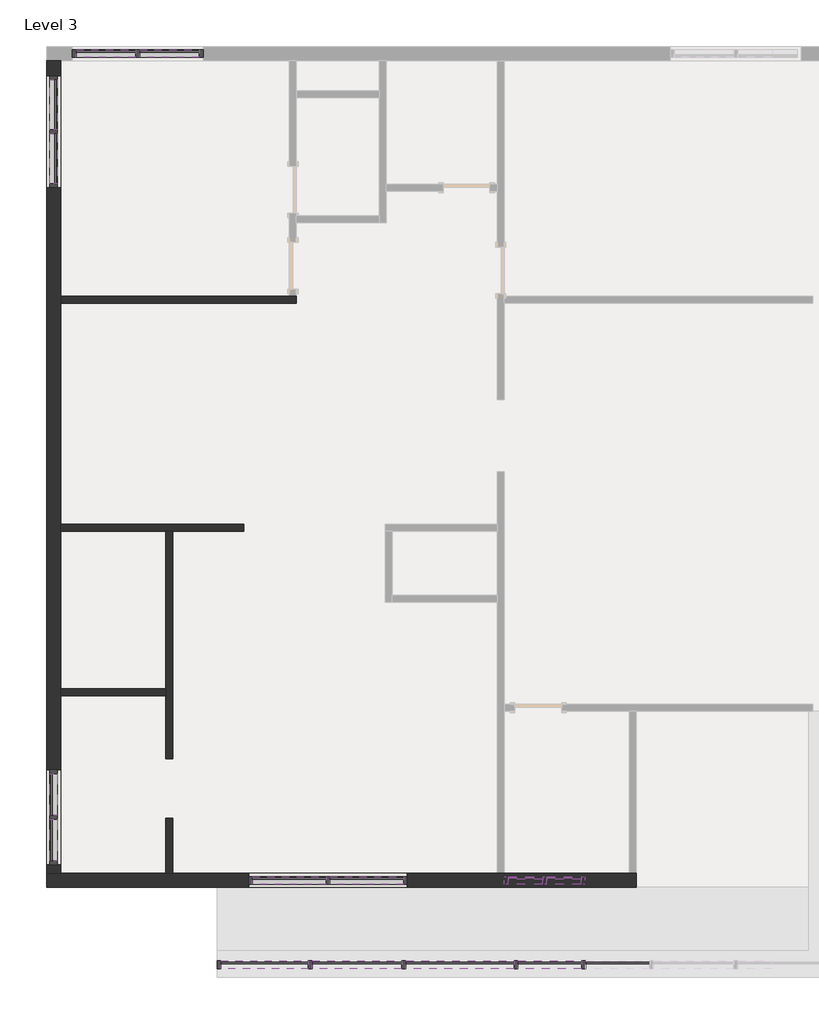
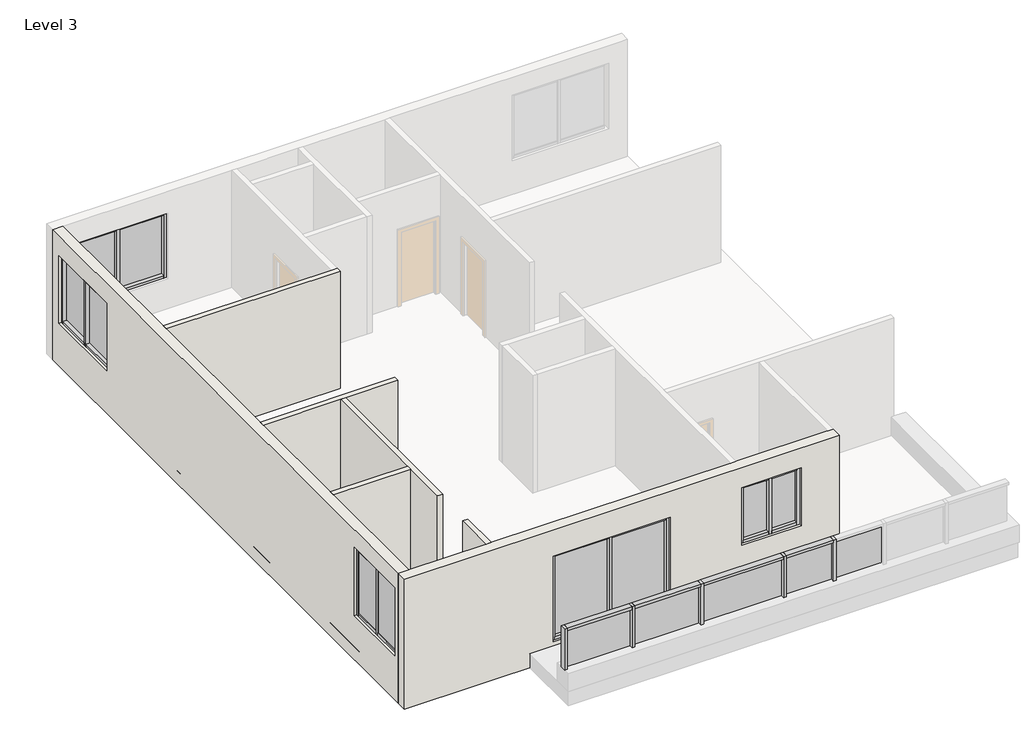
# One storey, part 1 of 2: 44 members, 15 plates, 7 walls.
"""IFC4 building model written with IfcOpenShell, lengths in millimetres."""

from ifc_helpers import new_model, si_unit, frame, origin, place, context, project, spatial, polyline, outline, extrude, faceted_brep, transform, mapped, element, save
from components import member_c17f1be2, member_801a2072, member_8e397d51, member_e9c7f4a4, member_4b34273c, member_2bcda102, member_43707fe5, member_d6231c0b, member_8613ee48, member_ea832cfd, member_e65a551c, member_6f41c4f0, member_2710255a, member_a910906a, member_01694e6c, member_4a1dde21, member_f8454dad, member_26d67f61, member_dda01c07, member_6d5c3e5e, member_04769ced, system_panel_glazed_e1e0096c, system_panel_glazed_c67bbfce, system_panel_glazed_bf6811db, system_panel_glazed_f54daf4a, system_panel_glazed_2cda0698, system_panel_glazed_7b3c61a9, system_panel_glazed_c86d0b30, system_panel_glazed_0021da76, system_panel_glazed_8b2f71d4

model = new_model("IFC4")

# Units and contexts
model_context = context("Model", 3, world=origin())
ifc_project = project(units=[si_unit("LENGTHUNIT", "METRE", prefix="MILLI")], contexts=[model_context])

# Site, building, storey
site = spatial("IfcSite", under=ifc_project)
building = spatial("IfcBuilding", under=site)
storey = spatial("IfcBuildingStorey", under=building, Name="Level 3", Elevation=6096.0)

# Members
placement = place(None, origin())
member_shape = member_c17f1be2(model_context)
element("IfcMember", 1, ObjectType="Rectangular Mullion : 2.5\" x 5\" rectangular", at=placement, inside=storey, context=model_context, shape_type="MappedRepresentation", body=[
    mapped(member_shape, transform((-18883.3195233, -1777.6752569, 8683.0746559), x_axis=(0.0, 0.0, 1.0), y_axis=(-1.0, 0.0, 0.0), z_axis=(0.0, -1.0, 0.0))),
])
element("IfcMember", 2, ObjectType="Rectangular Mullion : 2.5\" x 5\" rectangular", at=placement, inside=storey, context=model_context, shape_type="MappedRepresentation", body=[
    mapped(member_shape, transform((-18883.3195233, -2660.3252569, 8683.0746559), x_axis=(0.0, 0.0, 1.0), y_axis=(-1.0, 0.0, 0.0), z_axis=(0.0, -1.0, 0.0))),
])
element("IfcMember", 3, ObjectType="Rectangular Mullion : 2.5\" x 5\" rectangular", at=placement, inside=storey, context=model_context, shape_type="MappedRepresentation", body=[
    mapped(member_shape, transform((-18883.3195233, -1841.1752569, 7103.3616568), x_axis=(0.0, 0.0, -1.0), y_axis=(-1.0, 0.0, 0.0), z_axis=(0.0, 1.0, 0.0))),
])
element("IfcMember", 4, ObjectType="Rectangular Mullion : 2.5\" x 5\" rectangular", at=placement, inside=storey, context=model_context, shape_type="MappedRepresentation", body=[
    mapped(member_shape, transform((-18883.3195233, -958.5252569, 7103.3616568), x_axis=(0.0, 0.0, -1.0), y_axis=(-1.0, 0.0, 0.0), z_axis=(0.0, 1.0, 0.0))),
])
member_2_shape = member_801a2072(model_context)
element("IfcMember", 5, ObjectType="Rectangular Mullion : 2.5\" x 5\" rectangular", at=placement, inside=storey, context=model_context, shape_type="MappedRepresentation", body=[
    mapped(member_2_shape, transform((-17543.4695233, -533.0752569, 8635.8598955), x_axis=(0.0, 0.0, 1.0), y_axis=(0.0, -1.0, 0.0), z_axis=(1.0, 0.0, 0.0))),
])
element("IfcMember", 6, ObjectType="Rectangular Mullion : 2.5\" x 5\" rectangular", at=placement, inside=storey, context=model_context, shape_type="MappedRepresentation", body=[
    mapped(member_2_shape, transform((-16508.4195233, -533.0752569, 8635.8598955), x_axis=(0.0, 0.0, 1.0), y_axis=(0.0, -1.0, 0.0), z_axis=(1.0, 0.0, 0.0))),
])
element("IfcMember", 7, ObjectType="Rectangular Mullion : 2.5\" x 5\" rectangular", at=placement, inside=storey, context=model_context, shape_type="MappedRepresentation", body=[
    mapped(member_2_shape, transform((-17479.9695233, -533.0752569, 7102.6124164), x_axis=(0.0, 0.0, -1.0), y_axis=(0.0, -1.0, 0.0), z_axis=(-1.0, 0.0, 0.0))),
])
element("IfcMember", 8, ObjectType="Rectangular Mullion : 2.5\" x 5\" rectangular", at=placement, inside=storey, context=model_context, shape_type="MappedRepresentation", body=[
    mapped(member_2_shape, transform((-18515.0195233, -533.0752569, 7102.6124164), x_axis=(0.0, 0.0, -1.0), y_axis=(0.0, -1.0, 0.0), z_axis=(-1.0, 0.0, 0.0))),
])
member_3_shape = member_8e397d51(model_context)
element("IfcMember", 9, ObjectType="Rectangular Mullion : 2.5\" x 5\" rectangular", at=placement, inside=storey, context=model_context, shape_type="MappedRepresentation", body=[
    mapped(member_3_shape, transform((-10904.5445233, -14020.4752569, 8672.741835), x_axis=(0.0, 0.0, 1.0), y_axis=(0.0, -1.0, 0.0), z_axis=(1.0, 0.0, 0.0))),
])
element("IfcMember", 10, ObjectType="Rectangular Mullion : 2.5\" x 5\" rectangular", at=placement, inside=storey, context=model_context, shape_type="MappedRepresentation", body=[
    mapped(member_3_shape, transform((-10279.0695233, -14020.4752569, 8672.741835), x_axis=(0.0, 0.0, 1.0), y_axis=(0.0, -1.0, 0.0), z_axis=(1.0, 0.0, 0.0))),
])
element("IfcMember", 11, ObjectType="Rectangular Mullion : 2.5\" x 5\" rectangular", at=placement, inside=storey, context=model_context, shape_type="MappedRepresentation", body=[
    mapped(member_3_shape, transform((-10841.0445233, -14020.4752569, 7322.7664741), x_axis=(0.0, 0.0, -1.0), y_axis=(0.0, -1.0, 0.0), z_axis=(-1.0, 0.0, 0.0))),
])
element("IfcMember", 12, ObjectType="Rectangular Mullion : 2.5\" x 5\" rectangular", at=placement, inside=storey, context=model_context, shape_type="MappedRepresentation", body=[
    mapped(member_3_shape, transform((-11466.5195233, -14020.4752569, 7322.7664741), x_axis=(0.0, 0.0, -1.0), y_axis=(0.0, -1.0, 0.0), z_axis=(-1.0, 0.0, 0.0))),
])
member_4_shape = member_e9c7f4a4(model_context)
element("IfcMember", 13, ObjectType="Rectangular Mullion : 2.5\" x 5\" rectangular", at=placement, inside=storey, context=model_context, shape_type="MappedRepresentation", body=[
    mapped(member_4_shape, transform((-14438.3195233, -14020.4752569, 8530.8973501), x_axis=(0.0, 0.0, 1.0), y_axis=(0.0, -1.0, 0.0), z_axis=(1.0, 0.0, 0.0))),
])
element("IfcMember", 14, ObjectType="Rectangular Mullion : 2.5\" x 5\" rectangular", at=placement, inside=storey, context=model_context, shape_type="MappedRepresentation", body=[
    mapped(member_4_shape, transform((-13174.6695233, -14020.4752569, 8530.8973501), x_axis=(0.0, 0.0, 1.0), y_axis=(0.0, -1.0, 0.0), z_axis=(1.0, 0.0, 0.0))),
])
element("IfcMember", 15, ObjectType="Rectangular Mullion : 2.5\" x 5\" rectangular", at=placement, inside=storey, context=model_context, shape_type="MappedRepresentation", body=[
    mapped(member_4_shape, transform((-14374.8195233, -14020.4752569, 6521.4001776), x_axis=(0.0, 0.0, -1.0), y_axis=(0.0, -1.0, 0.0), z_axis=(-1.0, 0.0, 0.0))),
])
element("IfcMember", 16, ObjectType="Rectangular Mullion : 2.5\" x 5\" rectangular", at=placement, inside=storey, context=model_context, shape_type="MappedRepresentation", body=[
    mapped(member_4_shape, transform((-15638.4695233, -14020.4752569, 6521.4001776), x_axis=(0.0, 0.0, -1.0), y_axis=(0.0, -1.0, 0.0), z_axis=(-1.0, 0.0, 0.0))),
])
member_5_shape = member_4b34273c(model_context)
element("IfcMember", 17, ObjectType="Rectangular Mullion : 2.5\" x 5\" rectangular", at=placement, inside=storey, context=model_context, shape_type="MappedRepresentation", body=[
    mapped(member_5_shape, transform((-17511.7195233, -533.0752569, 7102.6124164), x_axis=(1.0, 0.0, 0.0), y_axis=(0.0, -1.0, 0.0), z_axis=(0.0, 0.0, -1.0))),
])
member_6_shape = member_2bcda102(model_context)
element("IfcMember", 18, ObjectType="Rectangular Mullion : 2.5\" x 5\" rectangular", at=placement, inside=storey, context=model_context, shape_type="MappedRepresentation", body=[
    mapped(member_6_shape, transform((-18578.5195233, -533.0752569, 8635.8598955), x_axis=(-1.0, 0.0, 0.0), y_axis=(0.0, -1.0, 0.0), z_axis=(0.0, 0.0, 1.0))),
])
element("IfcMember", 19, ObjectType="Rectangular Mullion : 2.5\" x 5\" rectangular", at=placement, inside=storey, context=model_context, shape_type="MappedRepresentation", body=[
    mapped(member_6_shape, transform((-16444.9195233, -533.0752569, 7102.6124164), x_axis=(1.0, 0.0, 0.0), y_axis=(0.0, -1.0, 0.0), z_axis=(0.0, 0.0, -1.0))),
])
member_7_shape = member_43707fe5(model_context)
element("IfcMember", 20, ObjectType="Rectangular Mullion : 2.5\" x 5\" rectangular", at=placement, inside=storey, context=model_context, shape_type="MappedRepresentation", body=[
    mapped(member_7_shape, transform((-18883.3195233, -1809.4252569, 7103.3616568), x_axis=(0.0, -1.0, 0.0), y_axis=(-1.0, 0.0, 0.0), z_axis=(0.0, 0.0, -1.0))),
])
member_8_shape = member_d6231c0b(model_context)
element("IfcMember", 21, ObjectType="Rectangular Mullion : 2.5\" x 5\" rectangular", at=placement, inside=storey, context=model_context, shape_type="MappedRepresentation", body=[
    mapped(member_8_shape, transform((-18883.3195233, -2723.8252569, 7103.3616568), x_axis=(0.0, -1.0, 0.0), y_axis=(-1.0, 0.0, 0.0), z_axis=(0.0, 0.0, -1.0))),
])
element("IfcMember", 22, ObjectType="Rectangular Mullion : 2.5\" x 5\" rectangular", at=placement, inside=storey, context=model_context, shape_type="MappedRepresentation", body=[
    mapped(member_8_shape, transform((-18883.3195233, -895.0252569, 8683.0746559), x_axis=(0.0, 1.0, 0.0), y_axis=(-1.0, 0.0, 0.0), z_axis=(0.0, 0.0, 1.0))),
])
member_9_shape = member_8613ee48(model_context)
element("IfcMember", 23, ObjectType="Rectangular Mullion : 2.5\" x 5\" rectangular", at=placement, inside=storey, context=model_context, shape_type="MappedRepresentation", body=[
    mapped(member_9_shape, transform((-18883.3195233, -13023.5252569, 8721.7723005), x_axis=(0.0, 0.0, 1.0), y_axis=(1.0, 0.0, 0.0), z_axis=(0.0, 1.0, 0.0))),
])
element("IfcMember", 24, ObjectType="Rectangular Mullion : 2.5\" x 5\" rectangular", at=placement, inside=storey, context=model_context, shape_type="MappedRepresentation", body=[
    mapped(member_9_shape, transform((-18883.3195233, -12280.5752569, 8721.7723005), x_axis=(0.0, 0.0, 1.0), y_axis=(1.0, 0.0, 0.0), z_axis=(0.0, 1.0, 0.0))),
])
member_10_shape = member_ea832cfd(model_context)
element("IfcMember", 25, ObjectType="Rectangular Mullion : 2.5\" x 5\" rectangular", at=placement, inside=storey, context=model_context, shape_type="MappedRepresentation", body=[
    mapped(member_10_shape, transform((-18883.3195233, -12991.7752569, 7128.502377), x_axis=(0.0, 1.0, 0.0), y_axis=(1.0, 0.0, 0.0), z_axis=(0.0, 0.0, -1.0))),
])
element("IfcMember", 26, ObjectType="Rectangular Mullion : 2.5\" x 5\" rectangular", at=placement, inside=storey, context=model_context, shape_type="MappedRepresentation", body=[
    mapped(member_9_shape, transform((-18883.3195233, -12960.0252569, 7128.502377), x_axis=(0.0, 0.0, -1.0), y_axis=(1.0, 0.0, 0.0), z_axis=(0.0, -1.0, 0.0))),
])
element("IfcMember", 27, ObjectType="Rectangular Mullion : 2.5\" x 5\" rectangular", at=placement, inside=storey, context=model_context, shape_type="MappedRepresentation", body=[
    mapped(member_9_shape, transform((-18883.3195233, -13702.9752569, 7128.502377), x_axis=(0.0, 0.0, -1.0), y_axis=(1.0, 0.0, 0.0), z_axis=(0.0, -1.0, 0.0))),
])
member_11_shape = member_e65a551c(model_context)
element("IfcMember", 28, ObjectType="Rectangular Mullion : 2.5\" x 5\" rectangular", at=placement, inside=storey, context=model_context, shape_type="MappedRepresentation", body=[
    mapped(member_11_shape, transform((-18883.3195233, -13766.4752569, 8721.7723005), x_axis=(0.0, -1.0, 0.0), y_axis=(1.0, 0.0, 0.0), z_axis=(0.0, 0.0, 1.0))),
])
element("IfcMember", 29, ObjectType="Rectangular Mullion : 2.5\" x 5\" rectangular", at=placement, inside=storey, context=model_context, shape_type="MappedRepresentation", body=[
    mapped(member_11_shape, transform((-18883.3195233, -12217.0752569, 7128.502377), x_axis=(0.0, 1.0, 0.0), y_axis=(1.0, 0.0, 0.0), z_axis=(0.0, 0.0, -1.0))),
])
member_12_shape = member_6f41c4f0(model_context)
element("IfcMember", 30, ObjectType="Rectangular Mullion : 2.5\" x 5\" rectangular", at=placement, inside=storey, context=model_context, shape_type="MappedRepresentation", body=[
    mapped(member_12_shape, transform((-14406.5695233, -14020.4752569, 6521.4001776), x_axis=(1.0, 0.0, 0.0), y_axis=(0.0, -1.0, 0.0), z_axis=(0.0, 0.0, -1.0))),
])
member_13_shape = member_2710255a(model_context)
element("IfcMember", 31, ObjectType="Rectangular Mullion : 2.5\" x 5\" rectangular", at=placement, inside=storey, context=model_context, shape_type="MappedRepresentation", body=[
    mapped(member_13_shape, transform((-13111.1695233, -14020.4752569, 6521.4001776), x_axis=(1.0, 0.0, 0.0), y_axis=(0.0, -1.0, 0.0), z_axis=(0.0, 0.0, -1.0))),
])
element("IfcMember", 32, ObjectType="Rectangular Mullion : 2.5\" x 5\" rectangular", at=placement, inside=storey, context=model_context, shape_type="MappedRepresentation", body=[
    mapped(member_13_shape, transform((-15701.9695233, -14020.4752569, 8530.8973501), x_axis=(-1.0, 0.0, 0.0), y_axis=(0.0, -1.0, 0.0), z_axis=(0.0, 0.0, 1.0))),
])
member_14_shape = member_a910906a(model_context)
element("IfcMember", 33, ObjectType="Rectangular Mullion : 2.5\" x 5\" rectangular", at=placement, inside=storey, context=model_context, shape_type="MappedRepresentation", body=[
    mapped(member_14_shape, transform((-10872.7945233, -14020.4752569, 7322.7664741), x_axis=(1.0, 0.0, 0.0), y_axis=(0.0, -1.0, 0.0), z_axis=(0.0, 0.0, -1.0))),
])
member_15_shape = member_01694e6c(model_context)
element("IfcMember", 34, ObjectType="Rectangular Mullion : 2.5\" x 5\" rectangular", at=placement, inside=storey, context=model_context, shape_type="MappedRepresentation", body=[
    mapped(member_15_shape, transform((-10215.5695233, -14020.4752569, 7322.7664741), x_axis=(1.0, 0.0, 0.0), y_axis=(0.0, -1.0, 0.0), z_axis=(0.0, 0.0, -1.0))),
])
element("IfcMember", 35, ObjectType="Rectangular Mullion : 2.5\" x 5\" rectangular", at=placement, inside=storey, context=model_context, shape_type="MappedRepresentation", body=[
    mapped(member_15_shape, transform((-11530.0195233, -14020.4752569, 8672.741835), x_axis=(-1.0, 0.0, 0.0), y_axis=(0.0, -1.0, 0.0), z_axis=(0.0, 0.0, 1.0))),
])
member_16_shape = member_4a1dde21(model_context)
element("IfcMember", 36, ObjectType="Rectangular Mullion : 2.5\" x 5\" rectangular", at=placement, inside=storey, context=model_context, shape_type="MappedRepresentation", body=[
    mapped(member_16_shape, transform((-13200.9712454, -15398.1130528, 7802.9269124), x_axis=(0.0, 0.0, 1.0), y_axis=(0.0, -1.0, 0.0), z_axis=(1.0, 0.0, 0.0))),
])
member_17_shape = member_f8454dad(model_context)
element("IfcMember", 37, ObjectType="Rectangular Mullion : 2.5\" x 5\" rectangular", at=placement, inside=storey, context=model_context, shape_type="MappedRepresentation", body=[
    mapped(member_17_shape, transform((-16217.2212454, -15398.1130528, 7802.9269124), x_axis=(-1.0, 0.0, 0.0), y_axis=(0.0, -1.0, 0.0), z_axis=(0.0, 0.0, 1.0))),
])
member_18_shape = member_26d67f61(model_context)
element("IfcMember", 38, ObjectType="Rectangular Mullion : 2.5\" x 5\" rectangular", at=placement, inside=storey, context=model_context, shape_type="MappedRepresentation", body=[
    mapped(member_18_shape, transform((-14724.9712454, -15398.1130528, 7802.9269124), x_axis=(0.0, 0.0, 1.0), y_axis=(0.0, -1.0, 0.0), z_axis=(1.0, 0.0, 0.0))),
])
member_19_shape = member_dda01c07(model_context)
element("IfcMember", 39, ObjectType="Rectangular Mullion : 2.5\" x 5\" rectangular", at=placement, inside=storey, context=model_context, shape_type="MappedRepresentation", body=[
    mapped(member_19_shape, transform((-14693.2212454, -15398.1130528, 6841.9204311), x_axis=(1.0, 0.0, 0.0), y_axis=(0.0, -1.0, 0.0), z_axis=(0.0, 0.0, -1.0))),
])
element("IfcMember", 40, ObjectType="Rectangular Mullion : 2.5\" x 5\" rectangular", at=placement, inside=storey, context=model_context, shape_type="MappedRepresentation", body=[
    mapped(member_19_shape, transform((-13169.2212454, -15398.1130528, 6841.9204311), x_axis=(1.0, 0.0, 0.0), y_axis=(0.0, -1.0, 0.0), z_axis=(0.0, 0.0, -1.0))),
])
element("IfcMember", 41, ObjectType="Rectangular Mullion : 2.5\" x 5\" rectangular", at=placement, inside=storey, context=model_context, shape_type="MappedRepresentation", body=[
    mapped(member_19_shape, transform((-11340.4212454, -15398.1130528, 6841.9204311), x_axis=(1.0, 0.0, 0.0), y_axis=(0.0, -1.0, 0.0), z_axis=(0.0, 0.0, -1.0))),
])
element("IfcMember", 42, ObjectType="Rectangular Mullion : 2.5\" x 5\" rectangular", at=placement, inside=storey, context=model_context, shape_type="MappedRepresentation", body=[
    mapped(member_19_shape, transform((-10235.0703844, -15398.1130528, 6841.9204311), x_axis=(1.0, 0.0, 0.0), y_axis=(0.0, -1.0, 0.0), z_axis=(0.0, 0.0, -1.0))),
])
member_20_shape = member_6d5c3e5e(model_context)
element("IfcMember", 43, ObjectType="Rectangular Mullion : 2.5\" x 5\" rectangular", at=placement, inside=storey, context=model_context, shape_type="MappedRepresentation", body=[
    mapped(member_20_shape, transform((-11372.1712454, -15398.1130528, 7802.9269124), x_axis=(0.0, 0.0, 1.0), y_axis=(0.0, -1.0, 0.0), z_axis=(1.0, 0.0, 0.0))),
])
member_21_shape = member_04769ced(model_context)
element("IfcMember", 44, ObjectType="Rectangular Mullion : 2.5\" x 5\" rectangular", at=placement, inside=storey, context=model_context, shape_type="MappedRepresentation", body=[
    mapped(member_21_shape, transform((-10266.8203844, -15398.1130528, 7802.9269124), x_axis=(0.0, 0.0, 1.0), y_axis=(0.0, -1.0, 0.0), z_axis=(1.0, 0.0, 0.0))),
])

# Plates
system_panel_glazed_shape = system_panel_glazed_e1e0096c(model_context)
element("IfcPlate", 45, ObjectType="System Panel : Glazed", at=placement, inside=storey, context=model_context, shape_type="MappedRepresentation", body=[
    mapped(system_panel_glazed_shape, transform((-18029.2445233, -533.0752569, 7166.1124164), x_axis=(1.0, 0.0, 0.0), y_axis=(0.0, 1.0, 0.0), z_axis=(0.0, 0.0, 1.0))),
])
element("IfcPlate", 46, ObjectType="System Panel : Glazed", at=placement, inside=storey, context=model_context, shape_type="MappedRepresentation", body=[
    mapped(system_panel_glazed_shape, transform((-16994.1945233, -533.0752569, 7166.1124164), x_axis=(1.0, 0.0, 0.0), y_axis=(0.0, 1.0, 0.0), z_axis=(0.0, 0.0, 1.0))),
])
system_panel_glazed_2_shape = system_panel_glazed_c67bbfce(model_context)
element("IfcPlate", 47, ObjectType="System Panel : Glazed", at=placement, inside=storey, context=model_context, shape_type="MappedRepresentation", body=[
    mapped(system_panel_glazed_2_shape, transform((-18883.3195233, -1368.1002569, 7166.8616568), x_axis=(0.0, -1.0, 0.0), y_axis=(1.0, 0.0, 0.0), z_axis=(0.0, 0.0, 1.0))),
])
element("IfcPlate", 48, ObjectType="System Panel : Glazed", at=placement, inside=storey, context=model_context, shape_type="MappedRepresentation", body=[
    mapped(system_panel_glazed_2_shape, transform((-18883.3195233, -2250.7502569, 7166.8616568), x_axis=(0.0, -1.0, 0.0), y_axis=(1.0, 0.0, 0.0), z_axis=(0.0, 0.0, 1.0))),
])
system_panel_glazed_3_shape = system_panel_glazed_bf6811db(model_context)
element("IfcPlate", 49, ObjectType="System Panel : Glazed", at=placement, inside=storey, context=model_context, shape_type="MappedRepresentation", body=[
    mapped(system_panel_glazed_3_shape, transform((-18883.3195233, -13363.2502569, 7192.002377), x_axis=(0.0, 1.0, 0.0), y_axis=(-1.0, 0.0, 0.0), z_axis=(0.0, 0.0, 1.0))),
])
element("IfcPlate", 50, ObjectType="System Panel : Glazed", at=placement, inside=storey, context=model_context, shape_type="MappedRepresentation", body=[
    mapped(system_panel_glazed_3_shape, transform((-18883.3195233, -12620.3002569, 7192.002377), x_axis=(0.0, 1.0, 0.0), y_axis=(-1.0, 0.0, 0.0), z_axis=(0.0, 0.0, 1.0))),
])
system_panel_glazed_4_shape = system_panel_glazed_f54daf4a(model_context)
element("IfcPlate", 51, ObjectType="System Panel : Glazed", at=placement, inside=storey, context=model_context, shape_type="MappedRepresentation", body=[
    mapped(system_panel_glazed_4_shape, transform((-15038.3945233, -14020.4752569, 6584.9001776), x_axis=(1.0, 0.0, 0.0), y_axis=(0.0, 1.0, 0.0), z_axis=(0.0, 0.0, 1.0))),
])
element("IfcPlate", 52, ObjectType="System Panel : Glazed", at=placement, inside=storey, context=model_context, shape_type="MappedRepresentation", body=[
    mapped(system_panel_glazed_4_shape, transform((-13774.7445233, -14020.4752569, 6584.9001776), x_axis=(1.0, 0.0, 0.0), y_axis=(0.0, 1.0, 0.0), z_axis=(0.0, 0.0, 1.0))),
])
system_panel_glazed_5_shape = system_panel_glazed_2cda0698(model_context)
element("IfcPlate", 53, ObjectType="System Panel : Glazed", at=placement, inside=storey, context=model_context, shape_type="MappedRepresentation", body=[
    mapped(system_panel_glazed_5_shape, transform((-11185.5320233, -14020.4752569, 7386.2664741), x_axis=(1.0, 0.0, 0.0), y_axis=(0.0, 1.0, 0.0), z_axis=(0.0, 0.0, 1.0))),
])
element("IfcPlate", 54, ObjectType="System Panel : Glazed", at=placement, inside=storey, context=model_context, shape_type="MappedRepresentation", body=[
    mapped(system_panel_glazed_5_shape, transform((-10560.0570233, -14020.4752569, 7386.2664741), x_axis=(1.0, 0.0, 0.0), y_axis=(0.0, 1.0, 0.0), z_axis=(0.0, 0.0, 1.0))),
])
system_panel_glazed_6_shape = system_panel_glazed_7b3c61a9(model_context)
element("IfcPlate", 55, ObjectType="System Panel : Glazed", at=placement, inside=storey, context=model_context, shape_type="MappedRepresentation", body=[
    mapped(system_panel_glazed_6_shape, transform((-15439.3462454, -15398.1130528, 6841.9204311), x_axis=(1.0, 0.0, 0.0), y_axis=(0.0, 1.0, 0.0), z_axis=(0.0, 0.0, 1.0))),
])
system_panel_glazed_7_shape = system_panel_glazed_c86d0b30(model_context)
element("IfcPlate", 56, ObjectType="System Panel : Glazed", at=placement, inside=storey, context=model_context, shape_type="MappedRepresentation", body=[
    mapped(system_panel_glazed_7_shape, transform((-13931.2212454, -15398.1130528, 6841.9204311), x_axis=(1.0, 0.0, 0.0), y_axis=(0.0, 1.0, 0.0), z_axis=(0.0, 0.0, 1.0))),
])
system_panel_glazed_8_shape = system_panel_glazed_0021da76(model_context)
element("IfcPlate", 57, ObjectType="System Panel : Glazed", at=placement, inside=storey, context=model_context, shape_type="MappedRepresentation", body=[
    mapped(system_panel_glazed_8_shape, transform((-12254.8212454, -15398.1130528, 6841.9204311), x_axis=(1.0, 0.0, 0.0), y_axis=(0.0, 1.0, 0.0), z_axis=(0.0, 0.0, 1.0))),
])
system_panel_glazed_9_shape = system_panel_glazed_8b2f71d4(model_context)
element("IfcPlate", 58, ObjectType="System Panel : Glazed", at=placement, inside=storey, context=model_context, shape_type="MappedRepresentation", body=[
    mapped(system_panel_glazed_9_shape, transform((-10787.7458149, -15398.1130528, 6841.9204311), x_axis=(1.0, 0.0, 0.0), y_axis=(0.0, 1.0, 0.0), z_axis=(0.0, 0.0, 1.0))),
])
element("IfcPlate", 59, ObjectType="System Panel : Glazed", at=placement, inside=storey, context=model_context, shape_type="MappedRepresentation", body=[
    mapped(system_panel_glazed_9_shape, transform((-9682.3949538, -15398.1130528, 6841.9204311), x_axis=(1.0, 0.0, 0.0), y_axis=(0.0, 1.0, 0.0), z_axis=(0.0, 0.0, 1.0))),
])

# Walls
element("IfcWall", 60, ObjectType="4.5\"", at=placement, inside=storey, context=model_context, shape_type="Brep", body=[
    faceted_brep([(-18769.0195233, -4609.7752569, 6096.0), (-14920.9195233, -4609.7752569, 6096.0), (-14920.9195233, -4609.7752569, 9144.0), (-18769.0195233, -4609.7752569, 9144.0), (-18769.0195233, -4495.4752569, 6096.0), (-18769.0195233, -4495.4752569, 9144.0), (-15035.2195233, -4495.4752569, 9144.0), (-14920.9195233, -4495.4752569, 9144.0), (-14920.9195233, -4495.4752569, 6096.0), (-15035.2195233, -4495.4752569, 6096.0)], [[[0, 1, 2, 3]], [[4, 5, 6, 7, 8, 9]], [[1, 0, 4, 9, 8]], [[3, 2, 7, 6, 5]], [[0, 3, 5, 4]], [[2, 1, 8, 7]]]),
])
element("IfcWall", 61, ObjectType="4.5\"", at=placement, inside=storey, context=model_context, shape_type="Brep", body=[
    faceted_brep([(-18769.0195233, -8324.5252569, 6096.0), (-17054.5195233, -8324.5252569, 6096.0), (-16940.2195233, -8324.5252569, 6096.0), (-15784.5195233, -8324.5252569, 6096.0), (-15784.5195233, -8324.5252569, 9144.0), (-16940.2195233, -8324.5252569, 9144.0), (-17054.5195233, -8324.5252569, 9144.0), (-18769.0195233, -8324.5252569, 9144.0), (-18769.0195233, -8210.2252569, 6096.0), (-18769.0195233, -8210.2252569, 9144.0), (-15784.5195233, -8210.2252569, 9144.0), (-15784.5195233, -8210.2252569, 6096.0)], [[[0, 1, 2, 3, 4, 5, 6, 7]], [[8, 9, 10, 11]], [[3, 2, 1, 0, 8, 11]], [[4, 3, 11, 10]], [[7, 6, 5, 4, 10, 9]], [[0, 7, 9, 8]]]),
])
element("IfcWall", 62, ObjectType="4.5\"", at=placement, inside=storey, context=model_context, shape_type="Brep", body=[
    faceted_brep([(-17054.5195233, -8324.5252569, 6096.0), (-17054.5195233, -10896.2752569, 6096.0), (-17054.5195233, -11010.5752569, 6096.0), (-17054.5195233, -12039.2752569, 6096.0), (-17054.5195233, -12039.2752569, 9144.0), (-17054.5195233, -11010.5752569, 9144.0), (-17054.5195233, -10896.2752569, 9144.0), (-17054.5195233, -8324.5252569, 9144.0), (-16940.2195233, -8324.5252569, 6096.0), (-16940.2195233, -8324.5252569, 9144.0), (-16940.2195233, -12039.2752569, 9144.0), (-16940.2195233, -12039.2752569, 6096.0)], [[[0, 1, 2, 3, 4, 5, 6, 7]], [[8, 9, 10, 11]], [[3, 2, 1, 0, 8, 11]], [[4, 3, 11, 10]], [[7, 6, 5, 4, 10, 9]], [[0, 7, 9, 8]]]),
])
element("IfcWall", 63, ObjectType="4.5\"", at=placement, inside=storey, context=model_context, shape_type="SweptSolid", body=[
    extrude(outline(polyline([(-17054.5195233, -11010.5752569), (-18769.0195233, -11010.5752569), (-18769.0195233, -10896.2752569), (-17054.5195233, -10896.2752569), (-17054.5195233, -11010.5752569)])), frame((0.0, 0.0, 6096.0), z_axis=(0.0, 0.0, 1.0), x_axis=(1.0, 0.0, 0.0)), (0.0, 0.0, 1.0), 3048.0),
])
element("IfcWall", 64, ObjectType="4.5\"", at=placement, inside=storey, context=model_context, shape_type="SweptSolid", body=[
    extrude(outline(polyline([(-16940.2195233, -13004.4752569), (-16940.2195233, -13906.1752569), (-17054.5195233, -13906.1752569), (-17054.5195233, -13004.4752569), (-16940.2195233, -13004.4752569)])), frame((0.0, 0.0, 6096.0), z_axis=(0.0, 0.0, 1.0), x_axis=(1.0, 0.0, 0.0)), (0.0, 0.0, 1.0), 3048.0),
])
element("IfcWall", 65, ObjectType="9\"", at=placement, inside=storey, context=model_context, shape_type="Brep", body=[
    faceted_brep([(-18769.0195233, -13906.1752569, 6096.0), (-18769.0195233, -11010.5752569, 6096.0), (-18769.0195233, -10896.2752569, 6096.0), (-18769.0195233, -8324.5252569, 6096.0), (-18769.0195233, -8210.2252569, 6096.0), (-18769.0195233, -4609.7752569, 6096.0), (-18769.0195233, -4495.4752569, 6096.0), (-18769.0195233, -647.3752569, 6096.0), (-18769.0195233, -647.3752569, 9144.0), (-18769.0195233, -4495.4752569, 9144.0), (-18769.0195233, -4609.7752569, 9144.0), (-18769.0195233, -8210.2252569, 9144.0), (-18769.0195233, -8324.5252569, 9144.0), (-18769.0195233, -10896.2752569, 9144.0), (-18769.0195233, -11010.5752569, 9144.0), (-18769.0195233, -13906.1752569, 9144.0), (-18769.0195233, -895.0252569, 8683.0746559), (-18769.0195233, -895.0252569, 7103.3616568), (-18769.0195233, -2723.8252569, 7103.3616568), (-18769.0195233, -2723.8252569, 8683.0746559), (-18769.0195233, -13766.4752569, 7128.502377), (-18769.0195233, -13766.4752569, 8721.7723005), (-18769.0195233, -12217.0752569, 8721.7723005), (-18769.0195233, -12217.0752569, 7128.502377), (-18997.6195233, -647.3752569, 6096.0), (-18997.6195233, -13906.1752569, 6096.0), (-18997.6195233, -13906.1752569, 9144.0), (-18997.6195233, -647.3752569, 9144.0), (-18997.6195233, -895.0252569, 7103.3616568), (-18997.6195233, -895.0252569, 8683.0746559), (-18997.6195233, -2723.8252569, 8683.0746559), (-18997.6195233, -2723.8252569, 7103.3616568), (-18997.6195233, -13766.4752569, 8721.7723005), (-18997.6195233, -13766.4752569, 7128.502377), (-18997.6195233, -12217.0752569, 7128.502377), (-18997.6195233, -12217.0752569, 8721.7723005)], [[[0, 1, 2, 3, 4, 5, 6, 7, 8, 9, 10, 11, 12, 13, 14, 15], [16, 17, 18, 19], [20, 21, 22, 23]], [[24, 25, 26, 27], [28, 29, 30, 31], [32, 33, 34, 35]], [[7, 6, 5, 4, 3, 2, 1, 0, 25, 24]], [[15, 14, 13, 12, 11, 10, 9, 8, 27, 26]], [[0, 15, 26, 25]], [[8, 7, 24, 27]], [[28, 17, 16, 29]], [[29, 16, 19, 30]], [[30, 19, 18, 31]], [[17, 28, 31, 18]], [[20, 33, 32, 21]], [[21, 32, 35, 22]], [[34, 23, 22, 35]], [[33, 20, 23, 34]]]),
])
element("IfcWall", 66, ObjectType="9\"", at=placement, inside=storey, context=model_context, shape_type="Brep", body=[
    faceted_brep([(-9377.3695233, -13906.1752569, 6096.0), (-9491.6695233, -13906.1752569, 6096.0), (-11530.0195233, -13906.1752569, 6096.0), (-11644.3195233, -13906.1752569, 6096.0), (-16940.2195233, -13906.1752569, 6096.0), (-17054.5195233, -13906.1752569, 6096.0), (-18769.0195233, -13906.1752569, 6096.0), (-18997.6195233, -13906.1752569, 6096.0), (-18997.6195233, -13906.1752569, 9144.0), (-18769.0195233, -13906.1752569, 9144.0), (-17054.5195233, -13906.1752569, 9144.0), (-16940.2195233, -13906.1752569, 9144.0), (-11644.3195233, -13906.1752569, 9144.0), (-11530.0195233, -13906.1752569, 9144.0), (-9491.6695233, -13906.1752569, 9144.0), (-9377.3695233, -13906.1752569, 9144.0), (-15701.9695233, -13906.1752569, 8530.8973501), (-15701.9695233, -13906.1752569, 6521.4001776), (-13111.1695233, -13906.1752569, 6521.4001776), (-13111.1695233, -13906.1752569, 8530.8973501), (-11530.0195233, -13906.1752569, 8672.741835), (-11530.0195233, -13906.1752569, 7322.7664741), (-10215.5695233, -13906.1752569, 7322.7664741), (-10215.5695233, -13906.1752569, 8672.741835), (-18997.6195233, -14134.7752569, 6096.0), (-9377.3695233, -14134.7752569, 6096.0), (-9377.3695233, -14134.7752569, 9144.0), (-18997.6195233, -14134.7752569, 9144.0), (-15701.9695233, -14134.7752569, 6521.4001776), (-15701.9695233, -14134.7752569, 8530.8973501), (-13111.1695233, -14134.7752569, 8530.8973501), (-13111.1695233, -14134.7752569, 6521.4001776), (-11530.0195233, -14134.7752569, 7322.7664741), (-11530.0195233, -14134.7752569, 8672.741835), (-10215.5695233, -14134.7752569, 8672.741835), (-10215.5695233, -14134.7752569, 7322.7664741)], [[[0, 1, 2, 3, 4, 5, 6, 7, 8, 9, 10, 11, 12, 13, 14, 15], [16, 17, 18, 19], [20, 21, 22, 23]], [[24, 25, 26, 27], [28, 29, 30, 31], [32, 33, 34, 35]], [[7, 6, 5, 4, 3, 2, 1, 0, 25, 24]], [[15, 14, 13, 12, 11, 10, 9, 8, 27, 26]], [[0, 15, 26, 25]], [[8, 7, 24, 27]], [[28, 17, 16, 29]], [[29, 16, 19, 30]], [[30, 19, 18, 31]], [[17, 28, 31, 18]], [[32, 21, 20, 33]], [[33, 20, 23, 34]], [[34, 23, 22, 35]], [[21, 32, 35, 22]]]),
])

save(model, "model.ifc")

# Revit data of these elements
# Type "Rectangular Mullion : 2.5\" x 5\" rectangular"
#   built-in parameter 1007304 = 0.416667 (stored number, unit not read)
#   built-in parameter 1007301 = 0.104167 (stored number, unit not read)
#   built-in parameter 1007300 = 0.104167 (stored number, unit not read)
# Type "System Panel : Glazed"
#   Construction Type Id = "GSP4R"
#   Analytic Construction = "1/8 in Pilkington single glazing"
#   Visual Light Transmittance = 0.9
#   Solar Heat Gain Coefficient = 0.86
#   Heat Transfer Coefficient (U) = 1.18115 BTU/(h·ft²·°F)
#   Define Thermal Properties by = 1
# Type "4.5\""
#   Assembly Code = "B2010"
#   Layers, outside or top first: 0' - 4 1/2" no material (function 1)
# Type "9\""
#   Assembly Code = "B2010"
#   Layers, outside or top first: 0' - 9" no material (function 1)
# Elements 1, 2, 3, 4, 5, 6, 7, 8, 9, 10, 11, 12, 13, 14, 15, 16, 17, 18, 19, 20, 21, 22, 23, 24, 25, 26, 27, 28, 29, 30, 31, 32, 33, 34, 35, 36, 37, 38, 39, 40, 41, 42, 43, 44 (IfcMember, "Rectangular Mullion : 2.5\" x 5\" rectangular")
#   Phase Created = New Construction
#   Materials on its faces: "Aluminum"
# Elements 45, 46, 47, 48, 49, 50, 51, 52, 53, 54, 55, 56, 57, 58, 59 (IfcPlate, "System Panel : Glazed")
#   Phase Created = New Construction
#   Materials on its faces: "Glass"
# Elements 60, 61, 62, 63, 64 (IfcWall, "4.5\"")
#   Top Offset = 0' - 0"
#   Base Offset = 0' - 0"
#   Unconnected Height = 10' - 0"
#   wall height = 10' - 0"
#   Phase Created = New Construction
#   Base Constraint = Level 3
#   Materials on its faces: "Default Wall"
# Elements 65, 66 (IfcWall, "9\"")
#   Top Offset = 0' - 0"
#   Base Offset = 0' - 0"
#   Unconnected Height = 10' - 0"
#   wall height = 10' - 0"
#   Phase Created = New Construction
#   Base Constraint = Level 3
#   Materials on its faces: "Default Wall"
# Materials
#   "Aluminum": class "Metal", colour RGB 247 247 247, transparency 0, Description = "Aluminum 6061", Cost = 0
#   "Glass": class "Glass", colour RGB 0 128 192, transparency 0.75, Description = "Soda Lime Glass", Cost = 0
#   "Default Wall": colour RGB 128 128 128, transparency 0, Cost = 0
